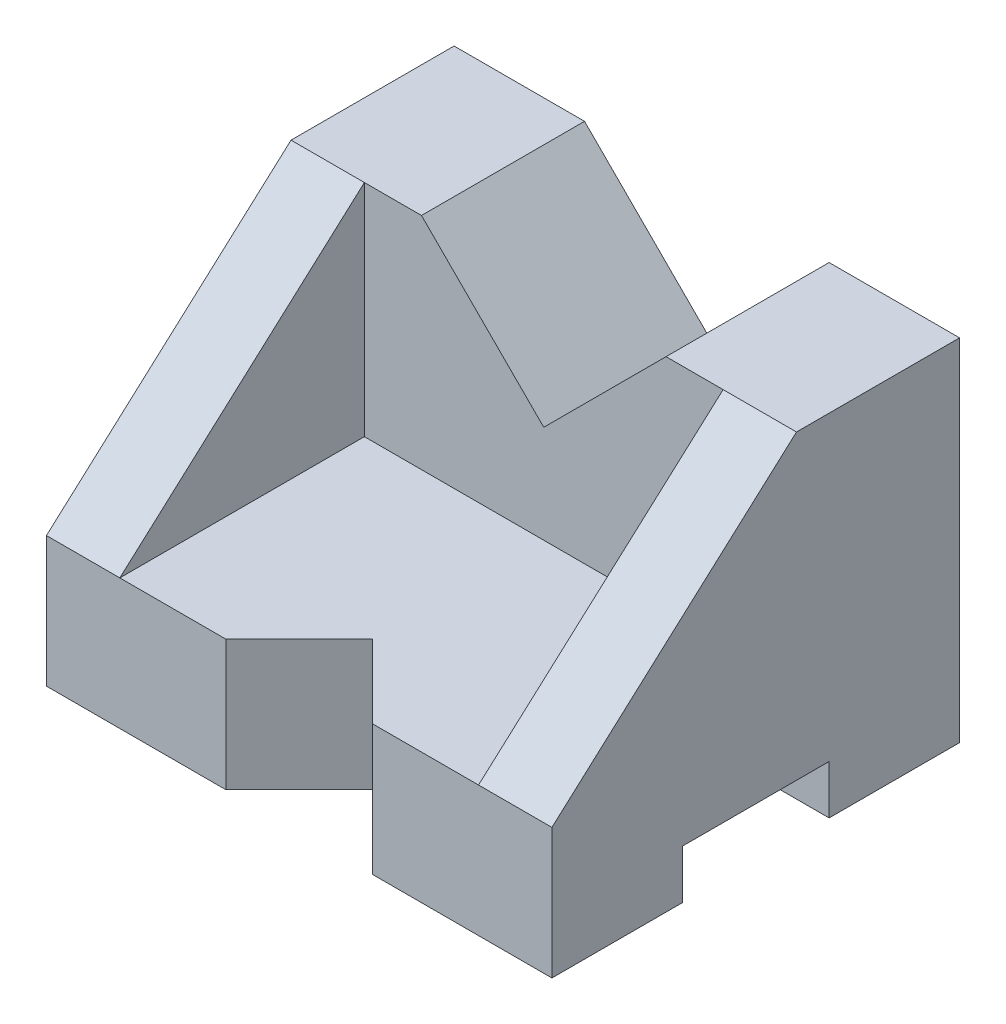
ISO-10303-21;
HEADER;
FILE_DESCRIPTION(('STEP AP214'),'2;1');
FILE_NAME('part.step','',(''),(''),'','','');
FILE_SCHEMA(('AUTOMOTIVE_DESIGN { 1 0 10303 214 1 1 1 1 }'));
ENDSEC;
DATA;
#1=APPLICATION_CONTEXT('core data for automotive mechanical design processes');
#2=APPLICATION_PROTOCOL_DEFINITION('international standard','automotive_design',2000,#1);
#3=PRODUCT_CONTEXT('',#1,'mechanical');
#4=PRODUCT('Part','Part','',(#3));
#5=PRODUCT_RELATED_PRODUCT_CATEGORY('part','',(#4));
#6=PRODUCT_DEFINITION_FORMATION('','',#4);
#7=PRODUCT_DEFINITION_CONTEXT('part definition',#1,'design');
#8=PRODUCT_DEFINITION('design','',#6,#7);
#9=PRODUCT_DEFINITION_SHAPE('','',#8);
#10=(LENGTH_UNIT() NAMED_UNIT(*) SI_UNIT(.MILLI.,.METRE.));
#11=(NAMED_UNIT(*) PLANE_ANGLE_UNIT() SI_UNIT($,.RADIAN.));
#12=(NAMED_UNIT(*) SI_UNIT($,.STERADIAN.) SOLID_ANGLE_UNIT());
#13=UNCERTAINTY_MEASURE_WITH_UNIT(LENGTH_MEASURE(1.E-05),#10,'distance_accuracy_value','');
#14=(GEOMETRIC_REPRESENTATION_CONTEXT(3) GLOBAL_UNCERTAINTY_ASSIGNED_CONTEXT((#13)) GLOBAL_UNIT_ASSIGNED_CONTEXT((#10,
#11,#12)) REPRESENTATION_CONTEXT('',''));
#15=CARTESIAN_POINT('',(0.,0.,0.));
#16=DIRECTION('',(0.,0.,1.));
#17=DIRECTION('',(1.,0.,0.));
#18=AXIS2_PLACEMENT_3D('',#15,#16,#17);
#19=CARTESIAN_POINT('',(0.,0.,100.));
#20=DIRECTION('',(0.,0.,1.));
#21=DIRECTION('',(1.,0.,0.));
#22=AXIS2_PLACEMENT_3D('',#19,#20,#21);
#23=PLANE('',#22);
#24=DIRECTION('',(0.,1.,0.));
#25=VECTOR('',#24,1.);
#26=CARTESIAN_POINT('',(-18.,-43.001,100.));
#27=LINE('',#26,#25);
#28=CARTESIAN_POINT('',(-18.,-43.,100.));
#29=VERTEX_POINT('',#28);
#30=CARTESIAN_POINT('',(-18.,-11.,100.));
#31=VERTEX_POINT('',#30);
#32=EDGE_CURVE('E171',#29,#31,#27,.T.);
#33=ORIENTED_EDGE('',*,*,#32,.T.);
#34=DIRECTION('',(-1.,0.,0.));
#35=VECTOR('',#34,1.);
#36=CARTESIAN_POINT('',(-44.,-11.,100.));
#37=LINE('',#36,#35);
#38=CARTESIAN_POINT('',(-44.,-11.,100.));
#39=VERTEX_POINT('',#38);
#40=EDGE_CURVE('E296',#31,#39,#37,.T.);
#41=ORIENTED_EDGE('',*,*,#40,.T.);
#42=DIRECTION('',(-1.,0.,0.));
#43=VECTOR('',#42,1.);
#44=CARTESIAN_POINT('',(62.,-11.,100.));
#45=LINE('',#44,#43);
#46=CARTESIAN_POINT('',(-62.,-11.,100.));
#47=VERTEX_POINT('',#46);
#48=EDGE_CURVE('E246',#39,#47,#45,.T.);
#49=ORIENTED_EDGE('',*,*,#48,.T.);
#50=DIRECTION('',(0.,-1.,0.));
#51=VECTOR('',#50,1.);
#52=CARTESIAN_POINT('',(-62.,-43.,100.));
#53=LINE('',#52,#51);
#54=CARTESIAN_POINT('',(-62.,-43.,100.));
#55=VERTEX_POINT('',#54);
#56=EDGE_CURVE('E190',#47,#55,#53,.T.);
#57=ORIENTED_EDGE('',*,*,#56,.T.);
#58=DIRECTION('',(1.,0.,0.));
#59=VECTOR('',#58,1.);
#60=CARTESIAN_POINT('',(-62.,-43.,100.));
#61=LINE('',#60,#59);
#62=EDGE_CURVE('E188',#55,#29,#61,.T.);
#63=ORIENTED_EDGE('',*,*,#62,.T.);
#64=EDGE_LOOP('',(#33,#41,#49,#57,#63));
#65=FACE_BOUND('',#64,.T.);
#66=ADVANCED_FACE('F39',(#65),#23,.T.);
#67=CARTESIAN_POINT('',(62.,43.,40.));
#68=DIRECTION('',(0.,-0.743294146247166,-0.66896473162245));
#69=DIRECTION('',(0.,0.66896473162245,-0.743294146247166));
#70=AXIS2_PLACEMENT_3D('',#67,#68,#69);
#71=PLANE('',#70);
#72=ORIENTED_EDGE('',*,*,#48,.F.);
#73=DIRECTION('',(0.,0.66896473162245,-0.743294146247166));
#74=VECTOR('',#73,1.);
#75=CARTESIAN_POINT('',(-44.,43.,40.));
#76=LINE('',#75,#74);
#77=CARTESIAN_POINT('',(-44.,43.,40.));
#78=VERTEX_POINT('',#77);
#79=EDGE_CURVE('E11',#39,#78,#76,.T.);
#80=ORIENTED_EDGE('',*,*,#79,.T.);
#81=DIRECTION('',(-1.,0.,0.));
#82=VECTOR('',#81,1.);
#83=CARTESIAN_POINT('',(62.,43.,40.));
#84=LINE('',#83,#82);
#85=CARTESIAN_POINT('',(-62.,43.,40.));
#86=VERTEX_POINT('',#85);
#87=EDGE_CURVE('E255',#78,#86,#84,.T.);
#88=ORIENTED_EDGE('',*,*,#87,.T.);
#89=DIRECTION('',(0.,-0.66896473162245,0.743294146247166));
#90=VECTOR('',#89,1.);
#91=CARTESIAN_POINT('',(-62.,43.,40.));
#92=LINE('',#91,#90);
#93=EDGE_CURVE('E253',#86,#47,#92,.T.);
#94=ORIENTED_EDGE('',*,*,#93,.T.);
#95=EDGE_LOOP('',(#72,#80,#88,#94));
#96=FACE_BOUND('',#95,.T.);
#97=ADVANCED_FACE('F359',(#96),#71,.F.);
#98=CARTESIAN_POINT('',(-62.,-43.,100.));
#99=DIRECTION('',(0.,1.,0.));
#100=DIRECTION('',(0.,0.,1.));
#101=AXIS2_PLACEMENT_3D('',#98,#99,#100);
#102=PLANE('',#101);
#103=DIRECTION('',(0.,0.,-1.));
#104=VECTOR('',#103,1.);
#105=CARTESIAN_POINT('',(62.,-43.,100.));
#106=LINE('',#105,#104);
#107=CARTESIAN_POINT('',(62.,-43.,32.));
#108=VERTEX_POINT('',#107);
#109=CARTESIAN_POINT('',(62.,-43.,0.));
#110=VERTEX_POINT('',#109);
#111=EDGE_CURVE('E225',#108,#110,#106,.T.);
#112=ORIENTED_EDGE('',*,*,#111,.F.);
#113=DIRECTION('',(-1.,0.,0.));
#114=VECTOR('',#113,1.);
#115=CARTESIAN_POINT('',(62.,-43.,32.));
#116=LINE('',#115,#114);
#117=CARTESIAN_POINT('',(-62.,-43.,32.));
#118=VERTEX_POINT('',#117);
#119=EDGE_CURVE('E262',#108,#118,#116,.T.);
#120=ORIENTED_EDGE('',*,*,#119,.T.);
#121=DIRECTION('',(0.,0.,-1.));
#122=VECTOR('',#121,1.);
#123=CARTESIAN_POINT('',(-62.,-43.,100.));
#124=LINE('',#123,#122);
#125=CARTESIAN_POINT('',(-62.,-43.,0.));
#126=VERTEX_POINT('',#125);
#127=EDGE_CURVE('E221',#118,#126,#124,.T.);
#128=ORIENTED_EDGE('',*,*,#127,.T.);
#129=DIRECTION('',(1.,0.,0.));
#130=VECTOR('',#129,1.);
#131=CARTESIAN_POINT('',(-62.,-43.,0.));
#132=LINE('',#131,#130);
#133=EDGE_CURVE('E216',#126,#110,#132,.T.);
#134=ORIENTED_EDGE('',*,*,#133,.T.);
#135=EDGE_LOOP('',(#112,#120,#128,#134));
#136=FACE_BOUND('',#135,.T.);
#137=ADVANCED_FACE('F331',(#136),#102,.F.);
#138=CARTESIAN_POINT('',(30.,43.,100.));
#139=DIRECTION('',(0.,-1.,0.));
#140=DIRECTION('',(0.,0.,-1.));
#141=AXIS2_PLACEMENT_3D('',#138,#139,#140);
#142=PLANE('',#141);
#143=DIRECTION('',(0.,0.,-1.));
#144=VECTOR('',#143,1.);
#145=CARTESIAN_POINT('',(30.,43.,100.));
#146=LINE('',#145,#144);
#147=CARTESIAN_POINT('',(30.,43.,40.));
#148=VERTEX_POINT('',#147);
#149=CARTESIAN_POINT('',(30.,43.,0.));
#150=VERTEX_POINT('',#149);
#151=EDGE_CURVE('E232',#148,#150,#146,.T.);
#152=ORIENTED_EDGE('',*,*,#151,.F.);
#153=DIRECTION('',(-1.,0.,0.));
#154=VECTOR('',#153,1.);
#155=CARTESIAN_POINT('',(-44.,43.,40.));
#156=LINE('',#155,#154);
#157=CARTESIAN_POINT('',(44.,43.,40.));
#158=VERTEX_POINT('',#157);
#159=EDGE_CURVE('E287',#158,#148,#156,.T.);
#160=ORIENTED_EDGE('',*,*,#159,.F.);
#161=CARTESIAN_POINT('',(62.,43.,40.));
#162=VERTEX_POINT('',#161);
#163=EDGE_CURVE('E242',#162,#158,#84,.T.);
#164=ORIENTED_EDGE('',*,*,#163,.F.);
#165=DIRECTION('',(0.,0.,-1.));
#166=VECTOR('',#165,1.);
#167=CARTESIAN_POINT('',(62.,43.,100.));
#168=LINE('',#167,#166);
#169=CARTESIAN_POINT('',(62.,43.,0.));
#170=VERTEX_POINT('',#169);
#171=EDGE_CURVE('E200',#162,#170,#168,.T.);
#172=ORIENTED_EDGE('',*,*,#171,.T.);
#173=DIRECTION('',(-1.,0.,0.));
#174=VECTOR('',#173,1.);
#175=CARTESIAN_POINT('',(30.,43.,0.));
#176=LINE('',#175,#174);
#177=EDGE_CURVE('E199',#170,#150,#176,.T.);
#178=ORIENTED_EDGE('',*,*,#177,.T.);
#179=EDGE_LOOP('',(#152,#160,#164,#172,#178));
#180=FACE_BOUND('',#179,.T.);
#181=ADVANCED_FACE('F41',(#180),#142,.F.);
#182=CARTESIAN_POINT('',(0.,13.,100.));
#183=DIRECTION('',(0.707106781186547,-0.707106781186548,0.));
#184=DIRECTION('',(0.707106781186548,0.707106781186547,0.));
#185=AXIS2_PLACEMENT_3D('',#182,#183,#184);
#186=PLANE('',#185);
#187=DIRECTION('',(0.,0.,-1.));
#188=VECTOR('',#187,1.);
#189=CARTESIAN_POINT('',(0.,13.,100.));
#190=LINE('',#189,#188);
#191=CARTESIAN_POINT('',(0.,13.,40.));
#192=VERTEX_POINT('',#191);
#193=CARTESIAN_POINT('',(0.,13.,0.));
#194=VERTEX_POINT('',#193);
#195=EDGE_CURVE('E235',#192,#194,#190,.T.);
#196=ORIENTED_EDGE('',*,*,#195,.F.);
#197=DIRECTION('',(0.707106781186548,0.707106781186547,0.));
#198=VECTOR('',#197,1.);
#199=CARTESIAN_POINT('',(0.,13.,40.));
#200=LINE('',#199,#198);
#201=EDGE_CURVE('E265',#192,#148,#200,.T.);
#202=ORIENTED_EDGE('',*,*,#201,.T.);
#203=ORIENTED_EDGE('',*,*,#151,.T.);
#204=DIRECTION('',(-0.707106781186548,-0.707106781186547,0.));
#205=VECTOR('',#204,1.);
#206=CARTESIAN_POINT('',(0.,13.,0.));
#207=LINE('',#206,#205);
#208=EDGE_CURVE('E201',#150,#194,#207,.T.);
#209=ORIENTED_EDGE('',*,*,#208,.T.);
#210=EDGE_LOOP('',(#196,#202,#203,#209));
#211=FACE_BOUND('',#210,.T.);
#212=ADVANCED_FACE('F349',(#211),#186,.F.);
#213=CARTESIAN_POINT('',(-30.,43.,100.));
#214=DIRECTION('',(-0.707106781186548,-0.707106781186547,0.));
#215=DIRECTION('',(0.707106781186547,-0.707106781186548,0.));
#216=AXIS2_PLACEMENT_3D('',#213,#214,#215);
#217=PLANE('',#216);
#218=DIRECTION('',(0.,0.,-1.));
#219=VECTOR('',#218,1.);
#220=CARTESIAN_POINT('',(-30.,43.,100.));
#221=LINE('',#220,#219);
#222=CARTESIAN_POINT('',(-30.,43.,40.));
#223=VERTEX_POINT('',#222);
#224=CARTESIAN_POINT('',(-30.,43.,0.));
#225=VERTEX_POINT('',#224);
#226=EDGE_CURVE('E230',#223,#225,#221,.T.);
#227=ORIENTED_EDGE('',*,*,#226,.F.);
#228=DIRECTION('',(0.707106781186547,-0.707106781186548,0.));
#229=VECTOR('',#228,1.);
#230=CARTESIAN_POINT('',(-30.,43.,40.));
#231=LINE('',#230,#229);
#232=EDGE_CURVE('E286',#223,#192,#231,.T.);
#233=ORIENTED_EDGE('',*,*,#232,.T.);
#234=ORIENTED_EDGE('',*,*,#195,.T.);
#235=DIRECTION('',(-0.707106781186547,0.707106781186548,0.));
#236=VECTOR('',#235,1.);
#237=CARTESIAN_POINT('',(-30.,43.,0.));
#238=LINE('',#237,#236);
#239=EDGE_CURVE('E210',#194,#225,#238,.T.);
#240=ORIENTED_EDGE('',*,*,#239,.T.);
#241=EDGE_LOOP('',(#227,#233,#234,#240));
#242=FACE_BOUND('',#241,.T.);
#243=ADVANCED_FACE('F352',(#242),#217,.F.);
#244=CARTESIAN_POINT('',(-62.,43.,100.));
#245=DIRECTION('',(0.,-1.,0.));
#246=DIRECTION('',(0.,0.,-1.));
#247=AXIS2_PLACEMENT_3D('',#244,#245,#246);
#248=PLANE('',#247);
#249=DIRECTION('',(0.,0.,-1.));
#250=VECTOR('',#249,1.);
#251=CARTESIAN_POINT('',(-62.,43.,100.));
#252=LINE('',#251,#250);
#253=CARTESIAN_POINT('',(-62.,43.,0.));
#254=VERTEX_POINT('',#253);
#255=EDGE_CURVE('E229',#86,#254,#252,.T.);
#256=ORIENTED_EDGE('',*,*,#255,.F.);
#257=ORIENTED_EDGE('',*,*,#87,.F.);
#258=EDGE_CURVE('E251',#223,#78,#84,.T.);
#259=ORIENTED_EDGE('',*,*,#258,.F.);
#260=ORIENTED_EDGE('',*,*,#226,.T.);
#261=DIRECTION('',(-1.,0.,0.));
#262=VECTOR('',#261,1.);
#263=CARTESIAN_POINT('',(-62.,43.,0.));
#264=LINE('',#263,#262);
#265=EDGE_CURVE('E209',#225,#254,#264,.T.);
#266=ORIENTED_EDGE('',*,*,#265,.T.);
#267=EDGE_LOOP('',(#256,#257,#259,#260,#266));
#268=FACE_BOUND('',#267,.T.);
#269=ADVANCED_FACE('F358',(#268),#248,.F.);
#270=CARTESIAN_POINT('',(-62.,-43.,100.));
#271=DIRECTION('',(1.,0.,0.));
#272=DIRECTION('',(0.,0.,-1.));
#273=AXIS2_PLACEMENT_3D('',#270,#271,#272);
#274=PLANE('',#273);
#275=ORIENTED_EDGE('',*,*,#127,.F.);
#276=DIRECTION('',(0.,-1.,0.));
#277=VECTOR('',#276,1.);
#278=CARTESIAN_POINT('',(-62.,-43.,32.));
#279=LINE('',#278,#277);
#280=CARTESIAN_POINT('',(-62.,-31.,32.));
#281=VERTEX_POINT('',#280);
#282=EDGE_CURVE('E245',#281,#118,#279,.T.);
#283=ORIENTED_EDGE('',*,*,#282,.F.);
#284=DIRECTION('',(0.,0.,-1.));
#285=VECTOR('',#284,1.);
#286=CARTESIAN_POINT('',(-62.,-31.,32.));
#287=LINE('',#286,#285);
#288=CARTESIAN_POINT('',(-62.,-31.,68.));
#289=VERTEX_POINT('',#288);
#290=EDGE_CURVE('E275',#289,#281,#287,.T.);
#291=ORIENTED_EDGE('',*,*,#290,.F.);
#292=DIRECTION('',(0.,1.,0.));
#293=VECTOR('',#292,1.);
#294=CARTESIAN_POINT('',(-62.,-43.,68.));
#295=LINE('',#294,#293);
#296=CARTESIAN_POINT('',(-62.,-43.,68.));
#297=VERTEX_POINT('',#296);
#298=EDGE_CURVE('E248',#297,#289,#295,.T.);
#299=ORIENTED_EDGE('',*,*,#298,.F.);
#300=EDGE_CURVE('E223',#55,#297,#124,.T.);
#301=ORIENTED_EDGE('',*,*,#300,.F.);
#302=ORIENTED_EDGE('',*,*,#56,.F.);
#303=ORIENTED_EDGE('',*,*,#93,.F.);
#304=ORIENTED_EDGE('',*,*,#255,.T.);
#305=DIRECTION('',(0.,-1.,0.));
#306=VECTOR('',#305,1.);
#307=CARTESIAN_POINT('',(-62.,-43.,0.));
#308=LINE('',#307,#306);
#309=EDGE_CURVE('E213',#254,#126,#308,.T.);
#310=ORIENTED_EDGE('',*,*,#309,.T.);
#311=EDGE_LOOP('',(#275,#283,#291,#299,#301,#302,#303,#304,#310));
#312=FACE_BOUND('',#311,.T.);
#313=ADVANCED_FACE('F325',(#312),#274,.F.);
#314=DIRECTION('',(0.707106781186548,0.,0.707106781186547));
#315=VECTOR('',#314,1.);
#316=CARTESIAN_POINT('',(0.,-43.,82.));
#317=LINE('',#316,#315);
#318=CARTESIAN_POINT('',(0.,-43.,82.));
#319=VERTEX_POINT('',#318);
#320=CARTESIAN_POINT('',(18.,-43.,100.));
#321=VERTEX_POINT('',#320);
#322=EDGE_CURVE('E162',#319,#321,#317,.T.);
#323=ORIENTED_EDGE('',*,*,#322,.F.);
#324=DIRECTION('',(0.707106781186547,0.,-0.707106781186548));
#325=VECTOR('',#324,1.);
#326=CARTESIAN_POINT('',(-18.,-43.,100.));
#327=LINE('',#326,#325);
#328=EDGE_CURVE('E309',#29,#319,#327,.T.);
#329=ORIENTED_EDGE('',*,*,#328,.F.);
#330=ORIENTED_EDGE('',*,*,#62,.F.);
#331=ORIENTED_EDGE('',*,*,#300,.T.);
#332=DIRECTION('',(-1.,0.,0.));
#333=VECTOR('',#332,1.);
#334=CARTESIAN_POINT('',(62.,-43.,68.));
#335=LINE('',#334,#333);
#336=CARTESIAN_POINT('',(62.,-43.,68.));
#337=VERTEX_POINT('',#336);
#338=EDGE_CURVE('E270',#337,#297,#335,.T.);
#339=ORIENTED_EDGE('',*,*,#338,.F.);
#340=CARTESIAN_POINT('',(62.,-43.,100.));
#341=VERTEX_POINT('',#340);
#342=EDGE_CURVE('E187',#341,#337,#106,.T.);
#343=ORIENTED_EDGE('',*,*,#342,.F.);
#344=EDGE_CURVE('E180',#321,#341,#61,.T.);
#345=ORIENTED_EDGE('',*,*,#344,.F.);
#346=EDGE_LOOP('',(#323,#329,#330,#331,#339,#343,#345));
#347=FACE_BOUND('',#346,.T.);
#348=ADVANCED_FACE('F184',(#347),#102,.F.);
#349=CARTESIAN_POINT('',(62.,-43.,100.));
#350=DIRECTION('',(-1.,0.,0.));
#351=DIRECTION('',(0.,0.,1.));
#352=AXIS2_PLACEMENT_3D('',#349,#350,#351);
#353=PLANE('',#352);
#354=DIRECTION('',(0.,0.,-1.));
#355=VECTOR('',#354,1.);
#356=CARTESIAN_POINT('',(62.,-31.,32.));
#357=LINE('',#356,#355);
#358=CARTESIAN_POINT('',(62.,-31.,68.));
#359=VERTEX_POINT('',#358);
#360=CARTESIAN_POINT('',(62.,-31.,32.));
#361=VERTEX_POINT('',#360);
#362=EDGE_CURVE('E62',#359,#361,#357,.T.);
#363=ORIENTED_EDGE('',*,*,#362,.T.);
#364=DIRECTION('',(0.,-1.,0.));
#365=VECTOR('',#364,1.);
#366=CARTESIAN_POINT('',(62.,-43.,32.));
#367=LINE('',#366,#365);
#368=EDGE_CURVE('E274',#361,#108,#367,.T.);
#369=ORIENTED_EDGE('',*,*,#368,.T.);
#370=ORIENTED_EDGE('',*,*,#111,.T.);
#371=DIRECTION('',(0.,1.,0.));
#372=VECTOR('',#371,1.);
#373=CARTESIAN_POINT('',(62.,-43.,0.));
#374=LINE('',#373,#372);
#375=EDGE_CURVE('E192',#110,#170,#374,.T.);
#376=ORIENTED_EDGE('',*,*,#375,.T.);
#377=ORIENTED_EDGE('',*,*,#171,.F.);
#378=DIRECTION('',(0.,-0.66896473162245,0.743294146247166));
#379=VECTOR('',#378,1.);
#380=CARTESIAN_POINT('',(62.,43.,40.));
#381=LINE('',#380,#379);
#382=CARTESIAN_POINT('',(62.,-11.,100.));
#383=VERTEX_POINT('',#382);
#384=EDGE_CURVE('E254',#162,#383,#381,.T.);
#385=ORIENTED_EDGE('',*,*,#384,.T.);
#386=DIRECTION('',(0.,1.,0.));
#387=VECTOR('',#386,1.);
#388=CARTESIAN_POINT('',(62.,-43.,100.));
#389=LINE('',#388,#387);
#390=EDGE_CURVE('E193',#341,#383,#389,.T.);
#391=ORIENTED_EDGE('',*,*,#390,.F.);
#392=ORIENTED_EDGE('',*,*,#342,.T.);
#393=DIRECTION('',(0.,1.,0.));
#394=VECTOR('',#393,1.);
#395=CARTESIAN_POINT('',(62.,-43.,68.));
#396=LINE('',#395,#394);
#397=EDGE_CURVE('E276',#337,#359,#396,.T.);
#398=ORIENTED_EDGE('',*,*,#397,.T.);
#399=EDGE_LOOP('',(#363,#369,#370,#376,#377,#385,#391,#392,#398));
#400=FACE_BOUND('',#399,.T.);
#401=ADVANCED_FACE('F324',(#400),#353,.F.);
#402=DIRECTION('',(0.,1.,0.));
#403=VECTOR('',#402,1.);
#404=CARTESIAN_POINT('',(18.,-43.001,100.));
#405=LINE('',#404,#403);
#406=CARTESIAN_POINT('',(18.,-11.,100.));
#407=VERTEX_POINT('',#406);
#408=EDGE_CURVE('E53',#321,#407,#405,.T.);
#409=ORIENTED_EDGE('',*,*,#408,.F.);
#410=ORIENTED_EDGE('',*,*,#344,.T.);
#411=ORIENTED_EDGE('',*,*,#390,.T.);
#412=CARTESIAN_POINT('',(44.,-11.,100.));
#413=VERTEX_POINT('',#412);
#414=EDGE_CURVE('E239',#383,#413,#45,.T.);
#415=ORIENTED_EDGE('',*,*,#414,.T.);
#416=EDGE_CURVE('E182',#413,#407,#37,.T.);
#417=ORIENTED_EDGE('',*,*,#416,.T.);
#418=EDGE_LOOP('',(#409,#410,#411,#415,#417));
#419=FACE_BOUND('',#418,.T.);
#420=ADVANCED_FACE('F175',(#419),#23,.T.);
#421=CARTESIAN_POINT('',(0.,0.,0.));
#422=DIRECTION('',(0.,0.,1.));
#423=DIRECTION('',(1.,0.,0.));
#424=AXIS2_PLACEMENT_3D('',#421,#422,#423);
#425=PLANE('',#424);
#426=ORIENTED_EDGE('',*,*,#177,.F.);
#427=ORIENTED_EDGE('',*,*,#375,.F.);
#428=ORIENTED_EDGE('',*,*,#133,.F.);
#429=ORIENTED_EDGE('',*,*,#309,.F.);
#430=ORIENTED_EDGE('',*,*,#265,.F.);
#431=ORIENTED_EDGE('',*,*,#239,.F.);
#432=ORIENTED_EDGE('',*,*,#208,.F.);
#433=EDGE_LOOP('',(#426,#427,#428,#429,#430,#431,#432));
#434=FACE_BOUND('',#433,.T.);
#435=ADVANCED_FACE('F340',(#434),#425,.F.);
#436=ORIENTED_EDGE('',*,*,#163,.T.);
#437=DIRECTION('',(0.,-0.66896473162245,0.743294146247166));
#438=VECTOR('',#437,1.);
#439=CARTESIAN_POINT('',(44.,43.,40.));
#440=LINE('',#439,#438);
#441=EDGE_CURVE('E50',#158,#413,#440,.T.);
#442=ORIENTED_EDGE('',*,*,#441,.T.);
#443=ORIENTED_EDGE('',*,*,#414,.F.);
#444=ORIENTED_EDGE('',*,*,#384,.F.);
#445=EDGE_LOOP('',(#436,#442,#443,#444));
#446=FACE_BOUND('',#445,.T.);
#447=ADVANCED_FACE('F236',(#446),#71,.F.);
#448=CARTESIAN_POINT('',(62.,-43.,32.));
#449=DIRECTION('',(0.,0.,-1.));
#450=DIRECTION('',(-1.,0.,0.));
#451=AXIS2_PLACEMENT_3D('',#448,#449,#450);
#452=PLANE('',#451);
#453=ORIENTED_EDGE('',*,*,#282,.T.);
#454=ORIENTED_EDGE('',*,*,#119,.F.);
#455=ORIENTED_EDGE('',*,*,#368,.F.);
#456=DIRECTION('',(-1.,0.,0.));
#457=VECTOR('',#456,1.);
#458=CARTESIAN_POINT('',(62.,-31.,32.));
#459=LINE('',#458,#457);
#460=EDGE_CURVE('E204',#361,#281,#459,.T.);
#461=ORIENTED_EDGE('',*,*,#460,.T.);
#462=EDGE_LOOP('',(#453,#454,#455,#461));
#463=FACE_BOUND('',#462,.T.);
#464=ADVANCED_FACE('F332',(#463),#452,.F.);
#465=CARTESIAN_POINT('',(62.,-31.,32.));
#466=DIRECTION('',(0.,1.,0.));
#467=DIRECTION('',(0.,0.,1.));
#468=AXIS2_PLACEMENT_3D('',#465,#466,#467);
#469=PLANE('',#468);
#470=ORIENTED_EDGE('',*,*,#290,.T.);
#471=ORIENTED_EDGE('',*,*,#460,.F.);
#472=ORIENTED_EDGE('',*,*,#362,.F.);
#473=DIRECTION('',(-1.,0.,0.));
#474=VECTOR('',#473,1.);
#475=CARTESIAN_POINT('',(62.,-31.,68.));
#476=LINE('',#475,#474);
#477=EDGE_CURVE('E267',#359,#289,#476,.T.);
#478=ORIENTED_EDGE('',*,*,#477,.T.);
#479=EDGE_LOOP('',(#470,#471,#472,#478));
#480=FACE_BOUND('',#479,.T.);
#481=ADVANCED_FACE('F330',(#480),#469,.F.);
#482=CARTESIAN_POINT('',(62.,-43.,68.));
#483=DIRECTION('',(0.,0.,1.));
#484=DIRECTION('',(1.,0.,0.));
#485=AXIS2_PLACEMENT_3D('',#482,#483,#484);
#486=PLANE('',#485);
#487=ORIENTED_EDGE('',*,*,#298,.T.);
#488=ORIENTED_EDGE('',*,*,#477,.F.);
#489=ORIENTED_EDGE('',*,*,#397,.F.);
#490=ORIENTED_EDGE('',*,*,#338,.T.);
#491=EDGE_LOOP('',(#487,#488,#489,#490));
#492=FACE_BOUND('',#491,.T.);
#493=ADVANCED_FACE('F326',(#492),#486,.F.);
#494=CARTESIAN_POINT('',(-44.,149.508215645555,100.));
#495=DIRECTION('',(-1.,0.,0.));
#496=DIRECTION('',(0.,0.,1.));
#497=AXIS2_PLACEMENT_3D('',#494,#495,#496);
#498=PLANE('',#497);
#499=DIRECTION('',(0.,0.,-1.));
#500=VECTOR('',#499,1.);
#501=CARTESIAN_POINT('',(-44.,-11.,100.));
#502=LINE('',#501,#500);
#503=CARTESIAN_POINT('',(-44.,-11.,40.));
#504=VERTEX_POINT('',#503);
#505=EDGE_CURVE('E168',#39,#504,#502,.T.);
#506=ORIENTED_EDGE('',*,*,#505,.T.);
#507=DIRECTION('',(0.,-1.,0.));
#508=VECTOR('',#507,1.);
#509=CARTESIAN_POINT('',(-44.,149.508215645555,40.));
#510=LINE('',#509,#508);
#511=EDGE_CURVE('E295',#78,#504,#510,.T.);
#512=ORIENTED_EDGE('',*,*,#511,.F.);
#513=ORIENTED_EDGE('',*,*,#79,.F.);
#514=EDGE_LOOP('',(#506,#512,#513));
#515=FACE_BOUND('',#514,.T.);
#516=ADVANCED_FACE('F365',(#515),#498,.F.);
#517=CARTESIAN_POINT('',(44.,149.508215645555,100.));
#518=DIRECTION('',(1.,0.,0.));
#519=DIRECTION('',(0.,0.,-1.));
#520=AXIS2_PLACEMENT_3D('',#517,#518,#519);
#521=PLANE('',#520);
#522=DIRECTION('',(0.,-1.,0.));
#523=VECTOR('',#522,1.);
#524=CARTESIAN_POINT('',(44.,149.508215645555,40.));
#525=LINE('',#524,#523);
#526=CARTESIAN_POINT('',(44.,-11.,40.));
#527=VERTEX_POINT('',#526);
#528=EDGE_CURVE('E292',#158,#527,#525,.T.);
#529=ORIENTED_EDGE('',*,*,#528,.T.);
#530=DIRECTION('',(0.,0.,1.));
#531=VECTOR('',#530,1.);
#532=CARTESIAN_POINT('',(44.,-11.,100.));
#533=LINE('',#532,#531);
#534=EDGE_CURVE('E297',#527,#413,#533,.T.);
#535=ORIENTED_EDGE('',*,*,#534,.T.);
#536=ORIENTED_EDGE('',*,*,#441,.F.);
#537=EDGE_LOOP('',(#529,#535,#536));
#538=FACE_BOUND('',#537,.T.);
#539=ADVANCED_FACE('F367',(#538),#521,.F.);
#540=CARTESIAN_POINT('',(-44.,149.508215645555,40.));
#541=DIRECTION('',(0.,0.,-1.));
#542=DIRECTION('',(-1.,0.,0.));
#543=AXIS2_PLACEMENT_3D('',#540,#541,#542);
#544=PLANE('',#543);
#545=ORIENTED_EDGE('',*,*,#232,.F.);
#546=ORIENTED_EDGE('',*,*,#258,.T.);
#547=ORIENTED_EDGE('',*,*,#511,.T.);
#548=DIRECTION('',(1.,0.,0.));
#549=VECTOR('',#548,1.);
#550=CARTESIAN_POINT('',(-44.,-11.,40.));
#551=LINE('',#550,#549);
#552=EDGE_CURVE('E298',#504,#527,#551,.T.);
#553=ORIENTED_EDGE('',*,*,#552,.T.);
#554=ORIENTED_EDGE('',*,*,#528,.F.);
#555=ORIENTED_EDGE('',*,*,#159,.T.);
#556=ORIENTED_EDGE('',*,*,#201,.F.);
#557=EDGE_LOOP('',(#545,#546,#547,#553,#554,#555,#556));
#558=FACE_BOUND('',#557,.T.);
#559=ADVANCED_FACE('F347',(#558),#544,.F.);
#560=CARTESIAN_POINT('',(0.,-11.,0.));
#561=DIRECTION('',(0.,-1.,0.));
#562=DIRECTION('',(0.,0.,-1.));
#563=AXIS2_PLACEMENT_3D('',#560,#561,#562);
#564=PLANE('',#563);
#565=ORIENTED_EDGE('',*,*,#40,.F.);
#566=DIRECTION('',(-0.707106781186547,0.,0.707106781186548));
#567=VECTOR('',#566,1.);
#568=CARTESIAN_POINT('',(-18.,-11.,100.));
#569=LINE('',#568,#567);
#570=CARTESIAN_POINT('',(0.,-11.,82.));
#571=VERTEX_POINT('',#570);
#572=EDGE_CURVE('E185',#571,#31,#569,.T.);
#573=ORIENTED_EDGE('',*,*,#572,.F.);
#574=DIRECTION('',(-0.707106781186548,0.,-0.707106781186547));
#575=VECTOR('',#574,1.);
#576=CARTESIAN_POINT('',(0.,-11.,82.));
#577=LINE('',#576,#575);
#578=EDGE_CURVE('E306',#407,#571,#577,.T.);
#579=ORIENTED_EDGE('',*,*,#578,.F.);
#580=ORIENTED_EDGE('',*,*,#416,.F.);
#581=ORIENTED_EDGE('',*,*,#534,.F.);
#582=ORIENTED_EDGE('',*,*,#552,.F.);
#583=ORIENTED_EDGE('',*,*,#505,.F.);
#584=EDGE_LOOP('',(#565,#573,#579,#580,#581,#582,#583));
#585=FACE_BOUND('',#584,.T.);
#586=ADVANCED_FACE('F370',(#585),#564,.F.);
#587=CARTESIAN_POINT('',(-18.,-43.001,100.));
#588=DIRECTION('',(-0.707106781186548,0.,-0.707106781186547));
#589=DIRECTION('',(-0.707106781186547,0.,0.707106781186548));
#590=AXIS2_PLACEMENT_3D('',#587,#588,#589);
#591=PLANE('',#590);
#592=ORIENTED_EDGE('',*,*,#328,.T.);
#593=DIRECTION('',(0.,1.,0.));
#594=VECTOR('',#593,1.);
#595=CARTESIAN_POINT('',(0.,-43.001,82.));
#596=LINE('',#595,#594);
#597=EDGE_CURVE('E164',#319,#571,#596,.T.);
#598=ORIENTED_EDGE('',*,*,#597,.T.);
#599=ORIENTED_EDGE('',*,*,#572,.T.);
#600=ORIENTED_EDGE('',*,*,#32,.F.);
#601=EDGE_LOOP('',(#592,#598,#599,#600));
#602=FACE_BOUND('',#601,.T.);
#603=ADVANCED_FACE('F315',(#602),#591,.F.);
#604=CARTESIAN_POINT('',(0.,-43.001,82.));
#605=DIRECTION('',(0.707106781186547,0.,-0.707106781186548));
#606=DIRECTION('',(-0.707106781186548,0.,-0.707106781186547));
#607=AXIS2_PLACEMENT_3D('',#604,#605,#606);
#608=PLANE('',#607);
#609=ORIENTED_EDGE('',*,*,#322,.T.);
#610=ORIENTED_EDGE('',*,*,#408,.T.);
#611=ORIENTED_EDGE('',*,*,#578,.T.);
#612=ORIENTED_EDGE('',*,*,#597,.F.);
#613=EDGE_LOOP('',(#609,#610,#611,#612));
#614=FACE_BOUND('',#613,.T.);
#615=ADVANCED_FACE('F163',(#614),#608,.F.);
#616=CLOSED_SHELL('',(#66,#97,#137,#181,#212,#243,#269,#313,#348,#401,#420,#435,#447,#464,#481,
#493,#516,#539,#559,#586,#603,#615));
#617=MANIFOLD_SOLID_BREP('B2',#616);
#618=ADVANCED_BREP_SHAPE_REPRESENTATION('',(#18,#617),#14);
#619=SHAPE_DEFINITION_REPRESENTATION(#9,#618);
ENDSEC;
END-ISO-10303-21;
